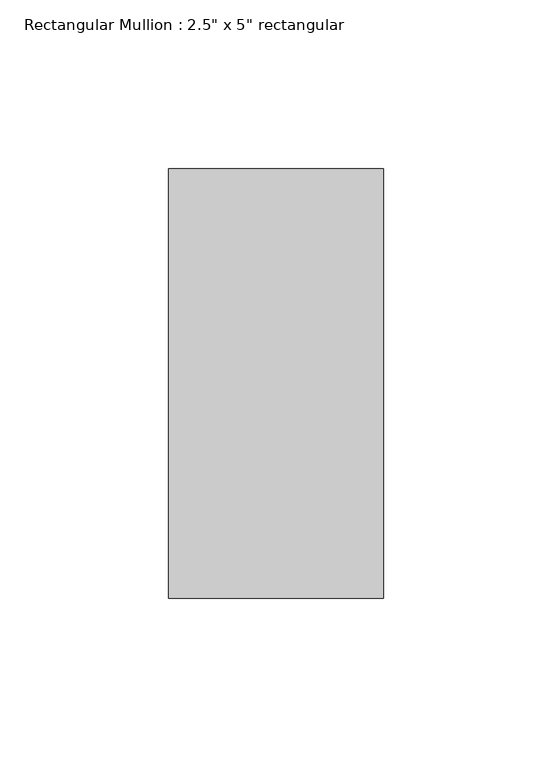
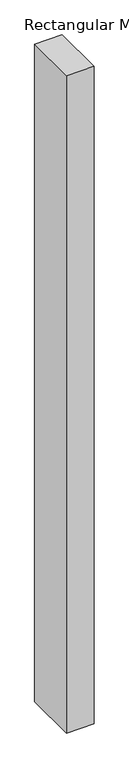
"""IFC4 building model written with IfcOpenShell, lengths in millimetres: member geometry."""

from ifc_helpers import new_model, si_unit, frame, origin, place, context, project, spatial, polyline, outline, extrude, source, transform, mapped, element, save


def member_b8b28852(model_context):
    return source(origin(), model_context, "Body", "SweptSolid", [
        extrude(outline(polyline([(31.75, 63.5), (31.75, -63.5), (-31.75, -63.5), (-31.75, 63.5), (31.75, 63.5)])), frame((0.0, 0.0, -1603.3915419), z_axis=(0.0, 0.0, 1.0), x_axis=(1.0, 0.0, 0.0)), (0.0, 0.0, 1.0), 1603.3915419),
    ])


if __name__ == "__main__":
    model = new_model("IFC4")
    model_context = context("Model", 3, world=origin())
    ifc_project = project(units=[si_unit("LENGTHUNIT", "METRE", prefix="MILLI")], contexts=[model_context])
    site = spatial("IfcSite", under=ifc_project)
    building = spatial("IfcBuilding", under=site)
    placement = place(None, origin())
    member_shape = member_b8b28852(model_context)
    element("IfcMember", 1, ObjectType="Rectangular Mullion : 2.5\" x 5\" rectangular", at=placement, inside=building, context=model_context, shape_type="MappedRepresentation", body=[
        mapped(member_shape, transform((0.0, 0.0, 0.0), x_axis=(1.0, 0.0, 0.0), y_axis=(0.0, 1.0, 0.0), z_axis=(0.0, 0.0, 1.0))),
    ])
    save(model, "model.ifc")

# Revit data of these elements
# Type "Rectangular Mullion : 2.5\" x 5\" rectangular"
#   built-in parameter 1007304 = 0.416667 (stored number, unit not read)
#   built-in parameter 1007301 = 0.104167 (stored number, unit not read)
#   built-in parameter 1007300 = 0.104167 (stored number, unit not read)
# Element 1 (IfcMember, "Rectangular Mullion : 2.5\" x 5\" rectangular")
#   Materials on its faces: "Aluminum"
# Materials
#   "Aluminum": class "Metal", colour RGB 247 247 247, transparency 0, Description = "Aluminum 6061", Cost = 0
